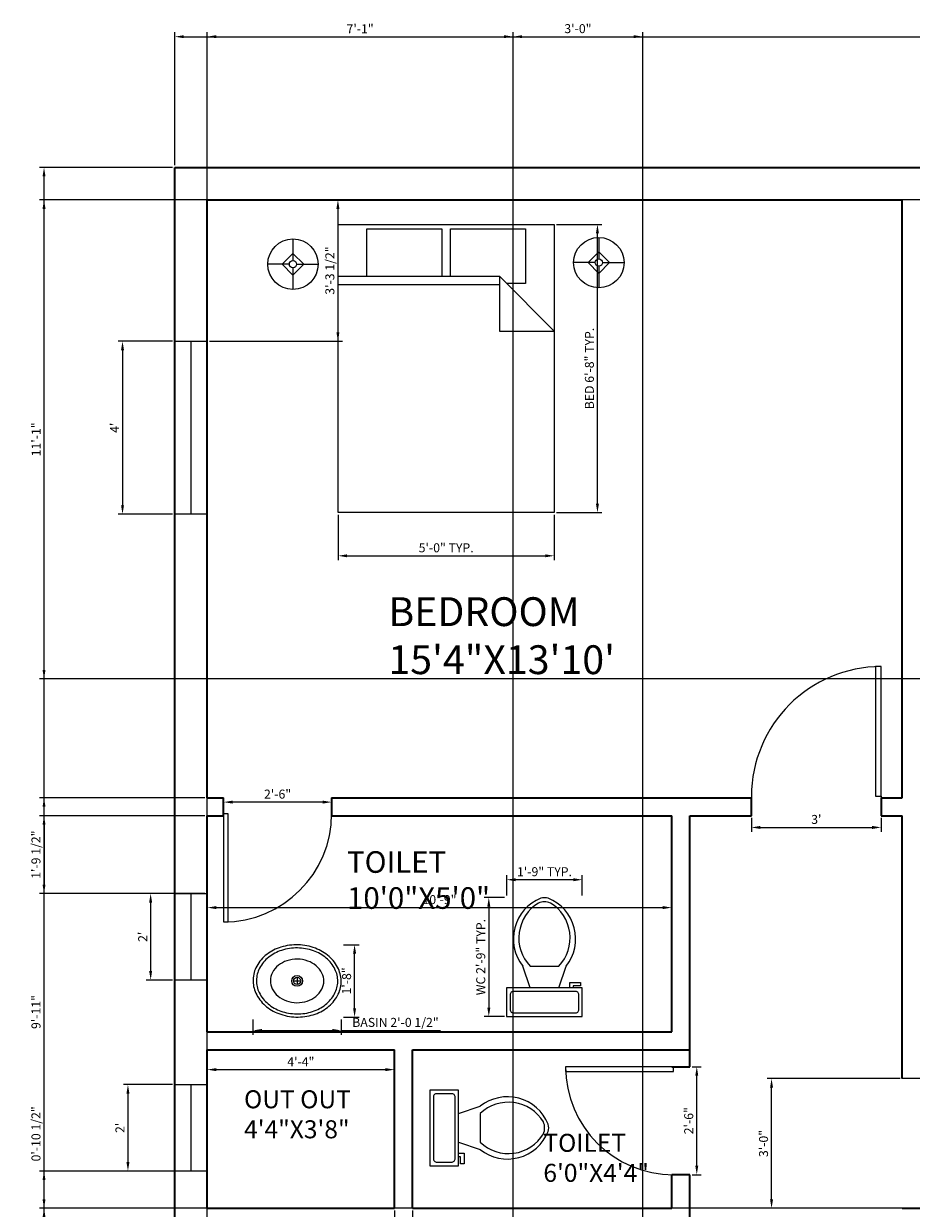
# Model space of a CAD drawing. Units: inches. Extents: x 3715 to 4224, y 2597 to 3354.
# Tile 4 of 5: x 3715 to 3961, y 3023 to 3352. Entities that reach past the tile are written whole.
import ezdxf

# ---------------------------------------------------------------- set-up
doc = ezdxf.new("R2010")
doc.units = ezdxf.units.IN
for name, color, linetype, lineweight in [('A-AREA-IDEN', 4, 'Continuous', 25), ('A-FLOR-FIXT', 9, 'Continuous', 18), ('A-WALL', 7, 'Continuous', 35), ('DIM', 1, 'Continuous', 18), ('DOOR', 3, 'Continuous', 25), ('FURNITURES', 30, 'Continuous', 18), ('WINDOW', 6, 'Continuous', 20)]:
    doc.layers.add(name, color=color, linetype=linetype, lineweight=lineweight)
doc.styles.get("Standard").update_dxf_attribs({"font": 'arial.ttf'})
doc.dimstyles.new('ISO-25', dxfattribs={"dimtxt": 2.5, "dimasz": 2.5, "dimexe": 1.25, "dimexo": 0.625, "dimtad": 1, "dimlunit": 3, "dimtxsty": 'Standard', "dimcen": 2.5, "dimadec": 0, "dimazin": 0, "dimtfac": 1, "dimtmove": 0, "dimatfit": 3, "dimfxl": 1, "dimarcsym": 0})

# ---------------------------------------------------------------- blocks, each defined once
blk = doc.blocks.new('*U4')
for p, q in [((0, 0), (0, -6)), ((-40, 0), (-40, -6))]:
    blk.add_line(p, q)
blk.add_lwpolyline([(0, 0), (0, 40), (-1.75, 40), (-1.75, 0)], close=True)
blk.add_arc((0, 0), 40, 90, 180)
blk = doc.blocks.new('*U5')
for p, q in [((0, 0), (0, 6)), ((40, 0), (40, 6))]:
    blk.add_line(p, q)
blk.add_lwpolyline([(0, 0), (0, -40), (1.75, -40), (1.75, 0)], close=True)
blk.add_arc((0, 0), 40, 270, 0)
blk = doc.blocks.new('Bed - Queen')
for p, q in [((0, -80.00003), (0, 0)), ((0, 0), (59.99999, 0)), ((59.99999, 0), (59.99999, -80.00003)), ((7.99999, -1.2), (28.79998, -1.2)), ((7.99999, -14.4), (7.99999, -1.2)), ((28.79998, -1.2), (28.79998, -14.4)), ((31.19999, -1.2), (51.99999, -1.2)), ((31.19999, -14.4), (31.19999, -1.2)), ((51.99999, -1.2), (51.99999, -16.4)), ((0, -14.4), (44.8, -14.4)), ((59.99999, -29.6), (44.8, -14.4)), ((44.8, -14.4), (44.8, -29.6)), ((51.99999, -16.4), (46.79936, -16.4)), ((44.8, -16.8), (0, -16.8)), ((44.8, -29.6), (59.99999, -29.6)), ((59.99999, -80.00003), (0, -80.00003))]:
    blk.add_line(p, q)
blk = doc.blocks.new('Lamp - Table')
for p, q in [((0, 7), (0, 1)), ((-1, 0), (-7, 0)), ((0, 3), (-3, 0)), ((-3, 0), (0, -3)), ((3, 0), (0, 3)), ((0, -3), (3, 0)), ((1, 0), (7, 0)), ((0, -1), (0, -7))]:
    blk.add_line(p, q)
for radius in [7, 1]:
    blk.add_circle((0, 0), radius)
blk = doc.blocks.new('Toilet - top')
for p, q in [((9.5, -6), (9.5, -2)), ((-10, -8.5), (-8, -8.5)), ((-10, -9.5), (-10, -8.5)), ((-7, -9.5), (-10, -9.5)), ((-8, -8.5), (-8, -8)), ((-7, -8), (-7, -9.5)), ((-4, -8), (-6, -14)), ((4, -8), (6, -14)), ((4, -14), (-4, -14))]:
    blk.add_line(p, q)
blk.add_lwpolyline([(10.5, -8), (10.5, 0), (-10.5, 0), (-10.5, -8)], close=True)
for points in [[(-9.5, -2), (-9.5, -6)], [(8.5, -1), (-8.5, -1)], [(-8.5, -7), (8.5, -7)]]:
    blk.add_lwpolyline(points)
for centre, radius, start, end in [((-8.62, -1.88), 0.884, 81.8699, 188.1301), ((8.62, -1.88), 0.884, 351.8699, 98.1301), ((-8.62, -6.12), 0.884, 171.8699, 278.1301), ((8.62, -6.12), 0.884, 261.8699, 8.1301), ((3.52, -21.58), 12.17, 141.4691, 247.9714), ((4.2, -21.82), 11.33, 136.3677, 238.9468), ((-3.52, -21.58), 12.17, 292.0284, 38.5307), ((-4.2, -21.82), 11.33, 301.053, 43.6321), ((0, -27.88), 4, 245.7318, 294.2682), ((0, -29), 4, 254.8605, 285.1395)]:
    blk.add_arc(centre, radius, start, end)
blk = doc.blocks.new('Sink - Oval top')
for p, q in [((-1, 0), (1, 0)), ((0, 1), (0, -1))]:
    blk.add_line(p, q)
for points in [[(-12.23, 0.39, 0.117634), (-11.46, -3.36, 0.104469), (-8.88, -6.8, 0.090016), (-5.08, -9.07, 0.08192), (-0.32, -10.02, 0.08192), (4.49, -9.38, 0.090016), (8.42, -7.36, 0.104469), (11.22, -4.09, 0.117634), (12.23, -0.39, 0.117634), (11.46, 3.36, 0.104469), (8.88, 6.8, 0.090016), (5.08, 9.07, 0.08192), (0.32, 10.02, 0.08192), (-4.49, 9.38, 0.090016), (-8.42, 7.36, 0.104469), (-11.22, 4.09, 0.117634)], [(-11.29, 0.16, 0.118622), (-10.52, -3.25, 0.104678), (-8.07, -6.36, 0.089562), (-4.54, -8.37, 0.081185), (-0.13, -9.15, 0.081185), (4.3, -8.49, 0.089562), (7.89, -6.58, 0.104678), (10.42, -3.55, 0.118622), (11.29, -0.16, 0.118622), (10.52, 3.25, 0.104678), (8.07, 6.36, 0.089562), (4.54, 8.37, 0.081185), (0.13, 9.15, 0.081185), (-4.3, 8.49, 0.089562), (-7.89, 6.58, 0.104678), (-10.42, 3.55, 0.118622)], [(-7.42, 0.08, 0.118283), (-6.91, -2.17, 0.104607), (-5.29, -4.21, 0.089718), (-2.97, -5.53, 0.081436), (-0.07, -6.04, 0.081436), (2.84, -5.59, 0.089718), (5.2, -4.33, 0.104607), (6.86, -2.32, 0.118283), (7.42, -0.08, 0.118283), (6.91, 2.17, 0.104607), (5.29, 4.21, 0.089718), (2.97, 5.53, 0.081436), (0.07, 6.04, 0.081436), (-2.84, 5.59, 0.089718), (-5.2, 4.33, 0.104607), (-6.86, 2.32, 0.118283)]]:
    blk.add_lwpolyline(points, format="xyb", close=True)
for radius in [1.5, 1]:
    blk.add_circle((0, 0), radius)
blk = doc.blocks.new('*D22')
at = {"layer": 'Defpoints', "color": 0, "transparency": 16777216}
for p in [(3756.48, 3263.65), (3741.97, 3215.65), (3756.48, 3215.65)]:
    blk.add_point(p, dxfattribs=at)
at = {"layer": 'DIM', "color": 0, "lineweight": -2, "transparency": 16777216}
for p, q in [((3755.85, 3263.65), (3740.72, 3263.65)), ((3741.97, 3261.15), (3741.97, 3218.15)), ((3755.85, 3215.65), (3740.72, 3215.65))]:
    blk.add_line(p, q, dxfattribs=at)
at = {"layer": 'DIM', "color": 0, "transparency": 16777216}
for points in [[(3741.55, 3261.15), (3742.39, 3261.15), (3741.97, 3263.65)], [(3741.55, 3218.15), (3742.39, 3218.15), (3741.97, 3215.65)]]:
    blk.add_solid(points, dxfattribs=at)
at = {"layer": 'DIM', "color": 0, "transparency": 16777216, "insert": (3740.1, 3239.65), "char_height": 2.5, "attachment_point": 5, "rotation": 90}
blk.add_mtext("4'", dxfattribs=at)
blk = doc.blocks.new('*D23')
at = {"layer": 'Defpoints', "color": 0, "transparency": 16777216}
for p in [(3756.48, 3110.32), (3749.78, 3086.32), (3756.48, 3086.32)]:
    blk.add_point(p, dxfattribs=at)
at = {"layer": 'DIM', "color": 0, "lineweight": -2, "transparency": 16777216}
for p, q in [((3755.85, 3110.32), (3748.53, 3110.32)), ((3749.78, 3107.82), (3749.78, 3088.82)), ((3755.85, 3086.32), (3748.53, 3086.32))]:
    blk.add_line(p, q, dxfattribs=at)
at = {"layer": 'DIM', "color": 0, "transparency": 16777216}
for points in [[(3749.36, 3107.82), (3750.19, 3107.82), (3749.78, 3110.32)], [(3749.36, 3088.82), (3750.19, 3088.82), (3749.78, 3086.32)]]:
    blk.add_solid(points, dxfattribs=at)
at = {"layer": 'DIM', "color": 0, "transparency": 16777216, "insert": (3747.9, 3098.32), "char_height": 2.5, "attachment_point": 5, "rotation": 90}
blk.add_mtext("2'", dxfattribs=at)
blk = doc.blocks.new('*D24')
at = {"layer": 'Defpoints', "color": 0, "transparency": 16777216}
for p in [(3756.48, 3057.27), (3743.47, 3033.27), (3756.48, 3033.27)]:
    blk.add_point(p, dxfattribs=at)
at = {"layer": 'DIM', "color": 0, "lineweight": -2, "transparency": 16777216}
for p, q in [((3755.85, 3057.27), (3742.22, 3057.27)), ((3743.47, 3054.77), (3743.47, 3035.77)), ((3755.85, 3033.27), (3742.22, 3033.27))]:
    blk.add_line(p, q, dxfattribs=at)
at = {"layer": 'DIM', "color": 0, "transparency": 16777216}
for points in [[(3743.06, 3054.77), (3743.89, 3054.77), (3743.47, 3057.27)], [(3743.06, 3035.77), (3743.89, 3035.77), (3743.47, 3033.27)]]:
    blk.add_solid(points, dxfattribs=at)
at = {"layer": 'DIM', "color": 0, "transparency": 16777216, "insert": (3741.59, 3045.27), "char_height": 2.5, "attachment_point": 5, "rotation": 90}
blk.add_mtext("2'", dxfattribs=at)
blk = doc.blocks.new('*D29')
at = {"layer": 'Defpoints', "color": 0, "transparency": 16777216}
for p in [(3765.48, 3066.93), (3817.48, 3064.87), (3817.48, 3061.44)]:
    blk.add_point(p, dxfattribs=at)
at = {"layer": 'DIM', "color": 0, "lineweight": -2, "transparency": 16777216}
for p, q in [((3765.48, 3066.31), (3765.48, 3060.19)), ((3817.48, 3064.25), (3817.48, 3060.19)), ((3767.98, 3061.44), (3814.98, 3061.44))]:
    blk.add_line(p, q, dxfattribs=at)
at = {"layer": 'DIM', "color": 0, "transparency": 16777216}
for points in [[(3767.98, 3061.86), (3767.98, 3061.02), (3765.48, 3061.44)], [(3814.98, 3061.86), (3814.98, 3061.02), (3817.48, 3061.44)]]:
    blk.add_solid(points, dxfattribs=at)
at = {"layer": 'DIM', "color": 0, "transparency": 16777216, "insert": (3791.48, 3063.31), "char_height": 2.5, "attachment_point": 5}
blk.add_mtext('4\'-4"', dxfattribs=at)
blk = doc.blocks.new('*D30')
at = {"layer": 'Defpoints', "color": 0, "transparency": 16777216}
for p in [(3894.48, 3106.42), (3765.48, 3071.93), (3894.48, 3071.93)]:
    blk.add_point(p, dxfattribs=at)
at = {"layer": 'DIM', "color": 0, "lineweight": -2, "transparency": 16777216}
for p, q in [((3765.48, 3072.56), (3765.48, 3107.67)), ((3767.98, 3106.42), (3891.98, 3106.42)), ((3894.48, 3072.56), (3894.48, 3107.67))]:
    blk.add_line(p, q, dxfattribs=at)
at = {"layer": 'DIM', "color": 0, "transparency": 16777216}
for points in [[(3767.98, 3106.84), (3767.98, 3106.01), (3765.48, 3106.42)], [(3891.98, 3106.84), (3891.98, 3106.01), (3894.48, 3106.42)]]:
    blk.add_solid(points, dxfattribs=at)
at = {"layer": 'DIM', "color": 0, "transparency": 16777216, "insert": (3829.98, 3108.32), "char_height": 2.5, "attachment_point": 5}
blk.add_mtext('10\'-9"', dxfattribs=at)
blk = doc.blocks.new('*D31')
at = {"layer": 'Defpoints', "color": 0, "transparency": 16777216}
for p in [(3916.6, 3131.93), (3952.6, 3131.93), (3952.6, 3128.68)]:
    blk.add_point(p, dxfattribs=at)
at = {"layer": 'DIM', "color": 0, "lineweight": -2, "transparency": 16777216}
for p, q in [((3916.6, 3131.31), (3916.6, 3127.43)), ((3952.6, 3131.31), (3952.6, 3127.43)), ((3919.1, 3128.68), (3950.1, 3128.68))]:
    blk.add_line(p, q, dxfattribs=at)
at = {"layer": 'DIM', "color": 0, "transparency": 16777216}
for points in [[(3919.1, 3129.1), (3919.1, 3128.26), (3916.6, 3128.68)], [(3950.1, 3129.1), (3950.1, 3128.26), (3952.6, 3128.68)]]:
    blk.add_solid(points, dxfattribs=at)
at = {"layer": 'DIM', "color": 0, "transparency": 16777216, "insert": (3934.6, 3130.58), "char_height": 2.5, "attachment_point": 5}
blk.add_mtext("3'", dxfattribs=at)
blk = doc.blocks.new('*D38')
at = {"layer": 'Defpoints', "color": 0, "transparency": 16777216}
for p in [(3899.48, 3062.26), (3901.41, 3062.26), (3899.48, 3032.26)]:
    blk.add_point(p, dxfattribs=at)
at = {"layer": 'DIM', "color": 0, "lineweight": -2, "transparency": 16777216}
for p, q in [((3900.1, 3062.26), (3902.66, 3062.26)), ((3901.41, 3034.76), (3901.41, 3059.76)), ((3900.1, 3032.26), (3902.66, 3032.26))]:
    blk.add_line(p, q, dxfattribs=at)
at = {"layer": 'DIM', "color": 0, "transparency": 16777216}
for points in [[(3900.99, 3059.76), (3901.82, 3059.76), (3901.41, 3062.26)], [(3900.99, 3034.76), (3901.82, 3034.76), (3901.41, 3032.26)]]:
    blk.add_solid(points, dxfattribs=at)
at = {"layer": 'DIM', "color": 0, "transparency": 16777216, "insert": (3899.5, 3047.26), "char_height": 2.5, "attachment_point": 5, "rotation": 90}
blk.add_mtext('2\'-6"', dxfattribs=at)
blk = doc.blocks.new('*D39')
at = {"layer": 'Defpoints', "color": 0, "transparency": 16777216}
for p in [(3770.02, 3136.93), (3770.02, 3135.71), (3800.02, 3136.93)]:
    blk.add_point(p, dxfattribs=at)
at = {"layer": 'DIM', "color": 0, "lineweight": -2, "transparency": 16777216}
for p, q in [((3770.02, 3136.31), (3770.02, 3134.46)), ((3797.52, 3135.71), (3772.52, 3135.71)), ((3800.02, 3136.31), (3800.02, 3134.46))]:
    blk.add_line(p, q, dxfattribs=at)
at = {"layer": 'DIM', "color": 0, "transparency": 16777216}
for points in [[(3772.52, 3136.13), (3772.52, 3135.3), (3770.02, 3135.71)], [(3797.52, 3136.13), (3797.52, 3135.3), (3800.02, 3135.71)]]:
    blk.add_solid(points, dxfattribs=at)
at = {"layer": 'DIM', "color": 0, "transparency": 16777216, "insert": (3785.02, 3137.61), "char_height": 2.5, "attachment_point": 5}
blk.add_mtext('2\'-6"', dxfattribs=at)
blk = doc.blocks.new('WIN-48IN-9IN-WALL')
blk.add_line((4.5, 48), (4.5, 0))
blk.add_lwpolyline([(0, 48), (9, 48), (9, 0), (0, 0)], close=True)
blk = doc.blocks.new('WIN-24IN-9IN-WALL')
blk.add_line((0, 4.5), (24, 4.5))
blk.add_lwpolyline([(0, 0), (0, 9), (24, 9), (24, 0)], close=True)
blk = doc.blocks.new('*D51')
at = {"layer": 'Defpoints', "color": 0, "transparency": 16777216}
for p in [(3861.83, 3296.1), (3873.83, 3296.1), (3861.83, 3216.1)]:
    blk.add_point(p, dxfattribs=at)
at = {"layer": 'DIM', "color": 0, "lineweight": -2, "transparency": 16777216}
for p, q in [((3862.46, 3296.1), (3875.08, 3296.1)), ((3873.83, 3218.6), (3873.83, 3293.6)), ((3862.46, 3216.1), (3875.08, 3216.1))]:
    blk.add_line(p, q, dxfattribs=at)
at = {"layer": 'DIM', "color": 0, "transparency": 16777216}
for points in [[(3873.41, 3293.6), (3874.25, 3293.6), (3873.83, 3296.1)], [(3873.41, 3218.6), (3874.25, 3218.6), (3873.83, 3216.1)]]:
    blk.add_solid(points, dxfattribs=at)
at = {"layer": 'DIM', "color": 0, "transparency": 16777216, "insert": (3871.93, 3256.1), "char_height": 2.5, "attachment_point": 5, "rotation": 90}
blk.add_mtext('BED 6\'-8" TYP.', dxfattribs=at)
blk = doc.blocks.new('*D52')
at = {"layer": 'Defpoints', "color": 0, "transparency": 16777216}
for p in [(3801.83, 3216.1), (3861.83, 3216.1), (3861.83, 3204.1)]:
    blk.add_point(p, dxfattribs=at)
at = {"layer": 'DIM', "color": 0, "lineweight": -2, "transparency": 16777216}
for p, q in [((3801.83, 3215.47), (3801.83, 3202.85)), ((3861.83, 3215.47), (3861.83, 3202.85)), ((3804.33, 3204.1), (3859.33, 3204.1))]:
    blk.add_line(p, q, dxfattribs=at)
at = {"layer": 'DIM', "color": 0, "transparency": 16777216}
for points in [[(3804.33, 3204.51), (3804.33, 3203.68), (3801.83, 3204.1)], [(3859.33, 3204.51), (3859.33, 3203.68), (3861.83, 3204.1)]]:
    blk.add_solid(points, dxfattribs=at)
at = {"layer": 'DIM', "color": 0, "transparency": 16777216, "insert": (3831.83, 3206), "char_height": 2.5, "attachment_point": 5}
blk.add_mtext('5\'-0" TYP.', dxfattribs=at)
blk = doc.blocks.new('*D55')
at = {"layer": 'Defpoints', "color": 0, "transparency": 16777216}
for p in [(3848.63, 3109.21), (3843.67, 3076.16), (3848.63, 3076.16)]:
    blk.add_point(p, dxfattribs=at)
at = {"layer": 'DIM', "color": 0, "lineweight": -2, "transparency": 16777216}
for p, q in [((3848, 3109.21), (3842.42, 3109.21)), ((3843.67, 3106.71), (3843.67, 3078.66)), ((3848, 3076.16), (3842.42, 3076.16))]:
    blk.add_line(p, q, dxfattribs=at)
at = {"layer": 'DIM', "color": 0, "transparency": 16777216}
for points in [[(3843.25, 3106.71), (3844.09, 3106.71), (3843.67, 3109.21)], [(3843.25, 3078.66), (3844.09, 3078.66), (3843.67, 3076.16)]]:
    blk.add_solid(points, dxfattribs=at)
at = {"layer": 'DIM', "color": 0, "transparency": 16777216, "insert": (3841.75, 3092.68), "char_height": 2.5, "attachment_point": 5, "rotation": 90}
blk.add_mtext('WC 2\'-9" TYP.', dxfattribs=at)
blk = doc.blocks.new('*D56')
at = {"layer": 'Defpoints', "color": 0, "transparency": 16777216}
for p in [(3848.63, 3114.16), (3848.63, 3109.21), (3869.63, 3109.21)]:
    blk.add_point(p, dxfattribs=at)
at = {"layer": 'DIM', "color": 0, "lineweight": -2, "transparency": 16777216}
for p, q in [((3848.63, 3109.83), (3848.63, 3115.41)), ((3869.63, 3109.83), (3869.63, 3115.41)), ((3867.13, 3114.16), (3851.13, 3114.16))]:
    blk.add_line(p, q, dxfattribs=at)
at = {"layer": 'DIM', "color": 0, "transparency": 16777216}
for points in [[(3851.13, 3114.58), (3851.13, 3113.75), (3848.63, 3114.16)], [(3867.13, 3114.58), (3867.13, 3113.75), (3869.63, 3114.16)]]:
    blk.add_solid(points, dxfattribs=at)
at = {"layer": 'DIM', "color": 0, "transparency": 16777216, "insert": (3859.13, 3116.07), "char_height": 2.5, "attachment_point": 5}
blk.add_mtext('1\'-9" TYP.', dxfattribs=at)
blk = doc.blocks.new('*D73')
at = {"layer": 'Defpoints', "color": 0, "transparency": 16777216}
for p in [(3778.17, 3076), (3802.72, 3076), (3802.72, 3072.31)]:
    blk.add_point(p, dxfattribs=at)
at = {"layer": 'DIM', "color": 0, "lineweight": -2, "transparency": 16777216}
for p, q in [((3778.17, 3075.37), (3778.17, 3071.06)), ((3802.72, 3075.37), (3802.72, 3071.06)), ((3780.67, 3072.31), (3800.22, 3072.31)), ((3802.72, 3072.31), (3830.28, 3072.31))]:
    blk.add_line(p, q, dxfattribs=at)
at = {"layer": 'DIM', "color": 0, "transparency": 16777216}
for points in [[(3780.67, 3072.73), (3780.67, 3071.9), (3778.17, 3072.31)], [(3800.22, 3072.73), (3800.22, 3071.9), (3802.72, 3072.31)]]:
    blk.add_solid(points, dxfattribs=at)
at = {"layer": 'DIM', "color": 0, "transparency": 16777216, "insert": (3817.75, 3074.23), "char_height": 2.5, "attachment_point": 5}
blk.add_mtext('BASIN 2\'-0 1/2"', dxfattribs=at)
blk = doc.blocks.new('*D74')
at = {"layer": 'Defpoints', "color": 0, "transparency": 16777216}
for p in [(3802.72, 3096.13), (3806.4, 3096.13), (3802.72, 3076)]:
    blk.add_point(p, dxfattribs=at)
at = {"layer": 'DIM', "color": 0, "lineweight": -2, "transparency": 16777216}
for p, q in [((3803.34, 3096.13), (3807.65, 3096.13)), ((3806.4, 3078.5), (3806.4, 3093.63)), ((3803.34, 3076), (3807.65, 3076))]:
    blk.add_line(p, q, dxfattribs=at)
at = {"layer": 'DIM', "color": 0, "transparency": 16777216}
for points in [[(3805.98, 3093.63), (3806.82, 3093.63), (3806.4, 3096.13)], [(3805.98, 3078.5), (3806.82, 3078.5), (3806.4, 3076)]]:
    blk.add_solid(points, dxfattribs=at)
at = {"layer": 'DIM', "color": 0, "transparency": 16777216, "insert": (3804.5, 3086.07), "char_height": 2.5, "attachment_point": 5, "rotation": 90}
blk.add_mtext('1\'-8"', dxfattribs=at)
blk = doc.blocks.new('*D75')
at = {"layer": 'Defpoints', "color": 0, "transparency": 16777216}
for p in [(4185.48, 3348.23), (3756.48, 3311.93), (4185.48, 3311.93)]:
    blk.add_point(p, dxfattribs=at)
at = {"layer": 'DIM', "color": 0, "lineweight": -2, "transparency": 16777216}
for p, q in [((3756.48, 3312.56), (3756.48, 3349.48)), ((4185.48, 3312.56), (4185.48, 3349.48)), ((3758.98, 3348.23), (4182.98, 3348.23))]:
    blk.add_line(p, q, dxfattribs=at)
at = {"layer": 'DIM', "color": 0, "transparency": 16777216}
for points in [[(3758.98, 3348.65), (3758.98, 3347.82), (3756.48, 3348.23)], [(4182.98, 3348.65), (4182.98, 3347.82), (4185.48, 3348.23)]]:
    blk.add_solid(points, dxfattribs=at)
at = {"layer": 'DIM', "color": 0, "transparency": 16777216, "insert": (3970.98, 3350.14), "char_height": 2.5, "attachment_point": 5}
blk.add_mtext('35\'-9"', dxfattribs=at)
blk = doc.blocks.new('*D76')
at = {"layer": 'Defpoints', "color": 0, "transparency": 16777216}
for p in [(3720.18, 3311.93), (3756.48, 3311.93), (3756.48, 2634.93)]:
    blk.add_point(p, dxfattribs=at)
at = {"layer": 'DIM', "color": 0, "lineweight": -2, "transparency": 16777216}
for p, q in [((3755.85, 3311.93), (3718.93, 3311.93)), ((3720.18, 2637.43), (3720.18, 3309.43)), ((3755.85, 2634.93), (3718.93, 2634.93))]:
    blk.add_line(p, q, dxfattribs=at)
at = {"layer": 'DIM', "color": 0, "transparency": 16777216}
for points in [[(3719.76, 3309.43), (3720.59, 3309.43), (3720.18, 3311.93)], [(3719.76, 2637.43), (3720.59, 2637.43), (3720.18, 2634.93)]]:
    blk.add_solid(points, dxfattribs=at)
at = {"layer": 'DIM', "color": 0, "transparency": 16777216, "insert": (3718.27, 2973.43), "char_height": 2.5, "attachment_point": 5, "rotation": 90}
blk.add_mtext('56\'-5"', dxfattribs=at)
blk = doc.blocks.new('*D77')
at = {"layer": 'Defpoints', "color": 0, "transparency": 16777216}
for p in [(3720.18, 3302.93), (4118.48, 3302.93), (4118.48, 3169.93)]:
    blk.add_point(p, dxfattribs=at)
at = {"layer": 'DIM', "color": 0, "lineweight": -2, "transparency": 16777216}
for p, q in [((4117.85, 3302.93), (3718.93, 3302.93)), ((3720.18, 3172.43), (3720.18, 3300.43)), ((4117.85, 3169.93), (3718.93, 3169.93))]:
    blk.add_line(p, q, dxfattribs=at)
at = {"layer": 'DIM', "color": 0, "transparency": 16777216}
for points in [[(3719.76, 3300.43), (3720.59, 3300.43), (3720.18, 3302.93)], [(3719.76, 3172.43), (3720.59, 3172.43), (3720.18, 3169.93)]]:
    blk.add_solid(points, dxfattribs=at)
at = {"layer": 'DIM', "color": 0, "transparency": 16777216, "insert": (3718.3, 3236.43), "char_height": 2.5, "attachment_point": 5, "rotation": 90}
blk.add_mtext('11\'-1"', dxfattribs=at)
blk = doc.blocks.new('*D79')
at = {"layer": 'Defpoints', "color": 0, "transparency": 16777216}
for p in [(3720.18, 3136.93), (3765.48, 3136.93), (3765.48, 3017.93)]:
    blk.add_point(p, dxfattribs=at)
at = {"layer": 'DIM', "color": 0, "lineweight": -2, "transparency": 16777216}
for p, q in [((3764.85, 3136.93), (3718.93, 3136.93)), ((3720.18, 3020.43), (3720.18, 3134.43)), ((3764.85, 3017.93), (3718.93, 3017.93))]:
    blk.add_line(p, q, dxfattribs=at)
at = {"layer": 'DIM', "color": 0, "transparency": 16777216}
for points in [[(3719.76, 3134.43), (3720.59, 3134.43), (3720.18, 3136.93)], [(3719.76, 3020.43), (3720.59, 3020.43), (3720.18, 3017.93)]]:
    blk.add_solid(points, dxfattribs=at)
at = {"layer": 'DIM', "color": 0, "transparency": 16777216, "insert": (3718.27, 3077.43), "char_height": 2.5, "attachment_point": 5, "rotation": 90}
blk.add_mtext('9\'-11"', dxfattribs=at)
blk = doc.blocks.new('*D83')
at = {"layer": 'Defpoints', "color": 0, "transparency": 16777216}
for p in [(3850.41, 3348.23), (3765.48, 2833.93), (3850.41, 2833.93)]:
    blk.add_point(p, dxfattribs=at)
at = {"layer": 'DIM', "color": 0, "lineweight": -2, "transparency": 16777216}
for p, q in [((3765.48, 2834.56), (3765.48, 3349.48)), ((3850.41, 2834.56), (3850.41, 3349.48)), ((3767.98, 3348.23), (3847.91, 3348.23))]:
    blk.add_line(p, q, dxfattribs=at)
at = {"layer": 'DIM', "color": 0, "transparency": 16777216}
for points in [[(3767.98, 3348.65), (3767.98, 3347.82), (3765.48, 3348.23)], [(3847.91, 3348.65), (3847.91, 3347.82), (3850.41, 3348.23)]]:
    blk.add_solid(points, dxfattribs=at)
at = {"layer": 'DIM', "color": 0, "transparency": 16777216, "insert": (3807.94, 3350.11), "char_height": 2.5, "attachment_point": 5}
blk.add_mtext('7\'-1"', dxfattribs=at)
blk = doc.blocks.new('*D84')
at = {"layer": 'Defpoints', "color": 0, "transparency": 16777216}
for p in [(3886.41, 3348.23), (3850.41, 2833.93), (3886.41, 2833.93)]:
    blk.add_point(p, dxfattribs=at)
at = {"layer": 'DIM', "color": 0, "lineweight": -2, "transparency": 16777216}
for p, q in [((3850.41, 2834.56), (3850.41, 3349.48)), ((3886.41, 2834.56), (3886.41, 3349.48)), ((3852.91, 3348.23), (3883.91, 3348.23))]:
    blk.add_line(p, q, dxfattribs=at)
at = {"layer": 'DIM', "color": 0, "transparency": 16777216}
for points in [[(3852.91, 3348.65), (3852.91, 3347.82), (3850.41, 3348.23)], [(3883.91, 3348.65), (3883.91, 3347.82), (3886.41, 3348.23)]]:
    blk.add_solid(points, dxfattribs=at)
at = {"layer": 'DIM', "color": 0, "transparency": 16777216, "insert": (3868.41, 3350.14), "char_height": 2.5, "attachment_point": 5}
blk.add_mtext('3\'-0"', dxfattribs=at)
blk = doc.blocks.new('*D85')
at = {"layer": 'Defpoints', "color": 0, "transparency": 16777216}
for p in [(3817.48, 3022.93), (3822.48, 3022.93), (3822.48, 2598.63)]:
    blk.add_point(p, dxfattribs=at)
at = {"layer": 'DIM', "color": 0, "lineweight": -2, "transparency": 16777216}
for p, q in [((3817.48, 3022.31), (3817.48, 2597.38)), ((3822.48, 3022.31), (3822.48, 2597.38)), ((3814.98, 2598.63), (3812.48, 2598.63)), ((3817.48, 2598.63), (3822.48, 2598.63)), ((3824.98, 2598.63), (3835.37, 2598.63))]:
    blk.add_line(p, q, dxfattribs=at)
at = {"layer": 'DIM', "color": 0, "transparency": 16777216}
for points in [[(3814.98, 2599.05), (3814.98, 2598.22), (3817.48, 2598.63)], [(3824.98, 2599.05), (3824.98, 2598.22), (3822.48, 2598.63)]]:
    blk.add_solid(points, dxfattribs=at)
at = {"layer": 'DIM', "color": 0, "transparency": 16777216, "insert": (3831.42, 2600.54), "char_height": 2.5, "attachment_point": 5}
blk.add_mtext('0\'-5"', dxfattribs=at)
blk = doc.blocks.new('*D90')
at = {"layer": 'Defpoints', "color": 0, "transparency": 16777216}
for p in [(3720.18, 3022.93), (3963.48, 3022.93), (3963.48, 3001.93)]:
    blk.add_point(p, dxfattribs=at)
at = {"layer": 'DIM', "color": 0, "lineweight": -2, "transparency": 16777216}
for p, q in [((3962.85, 3022.93), (3718.93, 3022.93)), ((3720.18, 3004.43), (3720.18, 3020.43)), ((3962.85, 3001.93), (3718.93, 3001.93))]:
    blk.add_line(p, q, dxfattribs=at)
at = {"layer": 'DIM', "color": 0, "transparency": 16777216}
for points in [[(3719.76, 3020.43), (3720.59, 3020.43), (3720.18, 3022.93)], [(3719.76, 3004.43), (3720.59, 3004.43), (3720.18, 3001.93)]]:
    blk.add_solid(points, dxfattribs=at)
at = {"layer": 'DIM', "color": 0, "transparency": 16777216, "insert": (3718.27, 3012.43), "char_height": 2.5, "attachment_point": 5, "rotation": 90}
blk.add_mtext('1\'-9"', dxfattribs=at)
blk = doc.blocks.new('*D91')
at = {"layer": 'Defpoints', "color": 0, "transparency": 16777216}
for p in [(3922.18, 3058.93), (3958.48, 3058.93), (3958.48, 3022.93)]:
    blk.add_point(p, dxfattribs=at)
at = {"layer": 'DIM', "color": 0, "lineweight": -2, "transparency": 16777216}
for p, q in [((3957.85, 3058.93), (3920.93, 3058.93)), ((3922.18, 3025.43), (3922.18, 3056.43)), ((3957.85, 3022.93), (3920.93, 3022.93))]:
    blk.add_line(p, q, dxfattribs=at)
at = {"layer": 'DIM', "color": 0, "transparency": 16777216}
for points in [[(3921.76, 3056.43), (3922.59, 3056.43), (3922.18, 3058.93)], [(3921.76, 3025.43), (3922.59, 3025.43), (3922.18, 3022.93)]]:
    blk.add_solid(points, dxfattribs=at)
at = {"layer": 'DIM', "color": 0, "transparency": 16777216, "insert": (3920.27, 3040.93), "char_height": 2.5, "attachment_point": 5, "rotation": 90}
blk.add_mtext('3\'-0"', dxfattribs=at)
blk = doc.blocks.new('*D97')
at = {"layer": 'Defpoints', "color": 0, "transparency": 16777216}
for p in [(3765.48, 3131.93), (3720.18, 3110.32), (3765.48, 3110.32)]:
    blk.add_point(p, dxfattribs=at)
at = {"layer": 'DIM', "color": 0, "lineweight": -2, "transparency": 16777216}
for p, q in [((3764.85, 3131.93), (3718.93, 3131.93)), ((3720.18, 3129.43), (3720.18, 3112.82)), ((3764.85, 3110.32), (3718.93, 3110.32))]:
    blk.add_line(p, q, dxfattribs=at)
at = {"layer": 'DIM', "color": 0, "transparency": 16777216}
for points in [[(3719.76, 3129.43), (3720.59, 3129.43), (3720.18, 3131.93)], [(3719.76, 3112.82), (3720.59, 3112.82), (3720.18, 3110.32)]]:
    blk.add_solid(points, dxfattribs=at)
at = {"layer": 'DIM', "color": 0, "transparency": 16777216, "insert": (3718.26, 3121.12), "char_height": 2.5, "attachment_point": 5, "rotation": 90}
blk.add_mtext('1\'-9 1/2"', dxfattribs=at)
blk = doc.blocks.new('*D98')
at = {"layer": 'Defpoints', "color": 0, "transparency": 16777216}
for p in [(3720.18, 3033.27), (3765.48, 3033.27), (3765.48, 3022.93)]:
    blk.add_point(p, dxfattribs=at)
at = {"layer": 'DIM', "color": 0, "lineweight": -2, "transparency": 16777216}
for p, q in [((3720.18, 3033.27), (3720.18, 3051.43)), ((3764.85, 3033.27), (3718.93, 3033.27)), ((3720.18, 3025.43), (3720.18, 3030.77)), ((3764.85, 3022.93), (3718.93, 3022.93))]:
    blk.add_line(p, q, dxfattribs=at)
at = {"layer": 'DIM', "color": 0, "transparency": 16777216}
for points in [[(3719.76, 3030.77), (3720.59, 3030.77), (3720.18, 3033.27)], [(3719.76, 3025.43), (3720.59, 3025.43), (3720.18, 3022.93)]]:
    blk.add_solid(points, dxfattribs=at)
at = {"layer": 'DIM', "color": 0, "transparency": 16777216, "insert": (3718.26, 3043.6), "char_height": 2.5, "attachment_point": 5, "rotation": 90}
blk.add_mtext('0\'-10 1/2"', dxfattribs=at)
blk = doc.blocks.new('*D100')
at = {"layer": 'Defpoints', "color": 0, "transparency": 16777216}
for p in [(3765.48, 3302.93), (3765.48, 3263.65), (3801.78, 3263.65)]:
    blk.add_point(p, dxfattribs=at)
at = {"layer": 'DIM', "color": 0, "lineweight": -2, "transparency": 16777216}
for p, q in [((3766.1, 3302.93), (3803.03, 3302.93)), ((3801.78, 3300.43), (3801.78, 3266.15)), ((3766.1, 3263.65), (3803.03, 3263.65))]:
    blk.add_line(p, q, dxfattribs=at)
at = {"layer": 'DIM', "color": 0, "transparency": 16777216}
for points in [[(3801.36, 3300.43), (3802.19, 3300.43), (3801.78, 3302.93)], [(3801.36, 3266.15), (3802.19, 3266.15), (3801.78, 3263.65)]]:
    blk.add_solid(points, dxfattribs=at)
at = {"layer": 'DIM', "color": 0, "transparency": 16777216, "insert": (3799.86, 3283.29), "char_height": 2.5, "attachment_point": 5, "rotation": 90}
blk.add_mtext('3\'-3 1/2"', dxfattribs=at)

msp = doc.modelspace()

# ---------------------------------------------------------------- linework, layer by layer
at = {"layer": 'A-WALL'}
for p, q in [((3756.476, 2634.934), (3756.476, 3311.934)), ((3756.476, 3311.934), (4185.476, 3311.934)), ((3765.476, 3302.934), (3958.476, 3302.934)), ((3765.476, 3136.934), (3765.476, 3302.934)), ((3958.476, 3136.934), (3958.476, 3302.934)), ((3765.476, 3136.934), (3770.02, 3136.934)), ((3800.02, 3136.934), (3916.604, 3136.934)), ((3952.604, 3136.934), (3958.476, 3136.934)), ((3765.476, 3131.934), (3770.02, 3131.934)), ((3765.476, 3071.934), (3765.476, 3131.934)), ((3800.02, 3131.934), (3894.476, 3131.934)), ((3894.476, 3071.934), (3894.476, 3131.934)), ((3899.476, 3062.26), (3899.476, 3131.934)), ((3899.476, 3131.934), (3916.604, 3131.934)), ((3952.604, 3131.934), (3958.476, 3131.934)), ((3958.476, 3058.934), (3958.476, 3131.934)), ((3765.476, 3071.934), (3894.476, 3071.934)), ((3765.476, 3066.934), (3817.476, 3066.934)), ((3765.476, 3022.934), (3765.476, 3066.934)), ((3817.476, 3022.934), (3817.476, 3066.934)), ((3822.476, 3022.934), (3822.476, 3066.934)), ((3822.476, 3066.934), (3899.476, 3066.934)), ((3894.476, 3022.934), (3894.476, 3032.26)), ((3899.476, 3017.934), (3899.476, 3032.26)), ((3765.476, 3022.934), (3817.476, 3022.934)), ((3822.476, 3022.934), (3894.476, 3022.934)), ((3958.476, 3022.934), (3963.476, 3022.934))]:
    msp.add_line(p, q, dxfattribs=at)
for points in [[(3770.02, 3131.934), (3770.02, 3136.934)], [(3800.02, 3136.934), (3800.02, 3131.934)], [(3916.604, 3131.934), (3916.604, 3136.934)], [(3952.604, 3136.934), (3952.604, 3131.934)], [(3894.476, 3062.26), (3899.476, 3062.26)], [(3899.476, 3032.26), (3894.476, 3032.26)]]:
    msp.add_lwpolyline(points, dxfattribs=at)

# ---------------------------------------------------------------- block references
at = {"layer": 'A-FLOR-FIXT'}
for p, rotation in [((3859.126, 3076.161), 180), ((3827.296, 3045.259), 89.99999999999999)]:
    msp.add_blockref('Toilet - top', p, dxfattribs=dict(at, rotation=rotation))
msp.add_blockref('Sink - Oval top', (3790.441, 3086.066), dxfattribs=at)
at = {"layer": 'DOOR'}
for name, p, xscale, yscale, zscale in [('*U4', (3952.604, 3137.334), 0.9, 0.9, 0.9), ('*U5', (3770.02, 3132.434), 0.75, 0.75, 0.75)]:
    msp.add_blockref(name, p, dxfattribs=dict(at, xscale=xscale, yscale=yscale, zscale=zscale))
for p, xscale, yscale, zscale, rotation in [((3894.976, 3062.26), 0.75, 0.75, 0.75, 90), ((3963.876, 3022.934), 0.9, 0.9, 0.9, 270)]:
    msp.add_blockref('*U4', p, dxfattribs=dict(at, xscale=xscale, yscale=yscale, zscale=zscale, rotation=rotation))
at = {"layer": 'FURNITURES'}
for name, p in [('Bed - Queen', (3801.832, 3296.096)), ('Lamp - Table', (3874.217, 3285.509)), ('Lamp - Table', (3789.286, 3285.062))]:
    msp.add_blockref(name, p, dxfattribs=at)
at = {"layer": 'WINDOW'}
msp.add_blockref('WIN-48IN-9IN-WALL', (3756.476, 3215.654), dxfattribs=at)
for p, rotation in [((3756.476, 3110.315), 269.999999999995), ((3756.476, 3057.27), 269.9999999999962)]:
    msp.add_blockref('WIN-24IN-9IN-WALL', p, dxfattribs=dict(at, rotation=rotation))

# ---------------------------------------------------------------- texts
at = {"layer": 'A-AREA-IDEN', "attachment_point": 1}
for s, insert, char_height in [('BEDROOM\\P15\'4"X13\'10\'', (3815.789, 3192.586), 8), ('TOILET\\P10\'0"X5\'0"', (3804.294, 3122.081), 6), ('OUT OUT\\P4\'4"X3\'8"', (3775.709, 3055.704), 5), ('TOILET\\P6\'0"X4\'4"', (3858.819, 3043.615), 5)]:
    msp.add_mtext_dynamic_manual_height_columns(s, width=94.29963, gutter_width=12.5, heights=[0], dxfattribs=dict(at, insert=insert, char_height=char_height))

# ---------------------------------------------------------------- dimensions: what is measured, and where the dimension line sits
at = {"layer": 'DIM'}
for base, p1, p2, override, picture, middle in [((4185.476, 3348.234), (3756.476, 3311.934), (4185.476, 3311.934), {"dimdec": 1, "dimlfac": 1, "dimrnd": 0, "dimzin": 1, "dimdsep": 46, "dimlunit": 4, "dimfrac": 2}, '*D75', (3970.976, 3350.136)), ((3850.407, 3348.234), (3765.476, 2833.934), (3850.407, 2833.934), {"dimdec": 1, "dimlfac": 1, "dimrnd": 0, "dimzin": 1, "dimdsep": 46, "dimlunit": 4, "dimfrac": 2}, '*D83', (3807.941, 3350.114)), ((3886.407, 3348.234), (3850.407, 2833.934), (3886.407, 2833.934), {"dimdec": 1, "dimlfac": 1, "dimrnd": 0, "dimzin": 1, "dimdsep": 46, "dimlunit": 4, "dimfrac": 2}, '*D84', (3868.407, 3350.136)), ((3770.02, 3135.713), (3800.02, 3136.934), (3770.02, 3136.934), {"dimclrd": 0, "dimclre": 0, "dimclrt": 0}, '*D39', (3785.02, 3137.614)), ((3952.604, 3128.68), (3916.604, 3131.934), (3952.604, 3131.934), {"dimclrd": 0, "dimclre": 0, "dimclrt": 0}, '*D31', (3934.604, 3130.582)), ((3894.476, 3106.422), (3765.476, 3071.934), (3894.476, 3071.934), {"dimclrd": 0, "dimclre": 0, "dimclrt": 0}, '*D30', (3829.976, 3108.324)), ((3817.476, 3061.439), (3765.476, 3066.934), (3817.476, 3064.87), {"dimclrd": 0, "dimclre": 0, "dimclrt": 0}, '*D29', (3791.476, 3063.314)), ((3822.476, 2598.634), (3817.476, 3022.934), (3822.476, 3022.934), {"dimdec": 1, "dimlfac": 1, "dimrnd": 0, "dimzin": 1, "dimdsep": 46, "dimlunit": 4, "dimfrac": 2}, '*D85', (3831.423, 2600.535))]:
    dim = msp.add_linear_dim(base=base, p1=p1, p2=p2, dimstyle='ISO-25', override=override, dxfattribs=at)
    dim.commit()
    dim.dimension.update_dxf_attribs({"geometry": picture, "text_midpoint": middle})
for base, p1, p2, angle, override, picture, middle in [((3720.176, 3311.934), (3756.476, 2634.934), (3756.476, 3311.934), 90, {"dimdec": 1, "dimlfac": 1, "dimrnd": 0, "dimzin": 1, "dimdsep": 46, "dimlunit": 4, "dimfrac": 2}, '*D76', (3718.274, 2973.434)), ((3720.176, 3302.934), (4118.476, 3169.934), (4118.476, 3302.934), 90, {"dimdec": 1, "dimlfac": 1, "dimrnd": 0, "dimzin": 1, "dimdsep": 46, "dimlunit": 4, "dimfrac": 2}, '*D77', (3718.295, 3236.434)), ((3801.776, 3263.654), (3765.476, 3302.934), (3765.476, 3263.654), 270, {"dimdec": 1, "dimlfac": 1, "dimrnd": 0, "dimzin": 1, "dimdsep": 46, "dimlunit": 4, "dimfrac": 2}, '*D100', (3799.857, 3283.294)), ((3741.971, 3215.654), (3756.476, 3263.654), (3756.476, 3215.654), 90, {"dimclrd": 0, "dimclre": 0, "dimclrt": 0}, '*D22', (3740.096, 3239.654)), ((3720.176, 3136.934), (3765.476, 3017.934), (3765.476, 3136.934), 90, {"dimdec": 1, "dimlfac": 1, "dimrnd": 0, "dimzin": 1, "dimdsep": 46, "dimlunit": 4, "dimfrac": 2}, '*D79', (3718.274, 3077.434)), ((3720.176, 3110.316), (3765.476, 3131.934), (3765.476, 3110.316), 90, {"dimdec": 1, "dimlfac": 1, "dimrnd": 0, "dimzin": 1, "dimdsep": 46, "dimlunit": 4, "dimfrac": 2}, '*D97', (3718.258, 3121.125)), ((3749.778, 3086.316), (3756.476, 3110.316), (3756.476, 3086.316), 90, {"dimclrd": 0, "dimclre": 0, "dimclrt": 0}, '*D23', (3747.898, 3098.316)), ((3806.399, 3096.134), (3802.716, 3075.997), (3802.716, 3096.134), 90, {"dimdec": 1, "dimlfac": 1, "dimrnd": 0, "dimzin": 1, "dimdsep": 46, "dimlunit": 4, "dimfrac": 2}, '*D74', (3804.497, 3086.066)), ((3901.406, 3062.26), (3899.476, 3032.26), (3899.476, 3062.26), 90, {"dimclrd": 0, "dimclre": 0, "dimclrt": 0}, '*D38', (3899.504, 3047.26)), ((3922.176, 3058.934), (3958.476, 3022.934), (3958.476, 3058.934), 90, {"dimdec": 1, "dimlfac": 1, "dimrnd": 0, "dimzin": 1, "dimdsep": 46, "dimlunit": 4, "dimfrac": 2}, '*D91', (3920.273, 3040.934)), ((3743.473, 3033.27), (3756.476, 3057.27), (3756.476, 3033.27), 90, {"dimclrd": 0, "dimclre": 0, "dimclrt": 0}, '*D24', (3741.593, 3045.27)), ((3720.176, 3033.27), (3765.476, 3022.934), (3765.476, 3033.27), 90, {"dimdec": 1, "dimlfac": 1, "dimrnd": 0, "dimzin": 1, "dimdsep": 46, "dimlunit": 4, "dimfrac": 2}, '*D98', (3718.258, 3043.602)), ((3720.176, 3022.934), (3963.476, 3001.934), (3963.476, 3022.934), 90, {"dimdec": 1, "dimlfac": 1, "dimrnd": 0, "dimzin": 1, "dimdsep": 46, "dimlunit": 4, "dimfrac": 2}, '*D90', (3718.274, 3012.434))]:
    dim = msp.add_linear_dim(base=base, p1=p1, p2=p2, angle=angle, dimstyle='ISO-25', override=override, dxfattribs=at)
    dim.commit()
    dim.dimension.update_dxf_attribs({"geometry": picture, "text_midpoint": middle})
for base, p1, p2, angle, text, picture, middle in [((3873.832, 3296.096), (3861.832, 3216.095), (3861.832, 3296.096), 90, 'BED <> TYP.', '*D51', (3871.93, 3256.095)), ((3848.626, 3114.164), (3869.626, 3109.207), (3848.626, 3109.207), 180, '<> TYP.', '*D56', (3859.126, 3116.065)), ((3843.669, 3076.161), (3848.626, 3109.207), (3848.626, 3076.161), 270, 'WC <> TYP.', '*D55', (3841.751, 3092.684))]:
    dim = msp.add_linear_dim(base=base, p1=p1, p2=p2, angle=angle, text=text, dimstyle='ISO-25', override={"dimdec": 1, "dimlfac": 1, "dimrnd": 0, "dimzin": 1, "dimdsep": 46, "dimlunit": 4, "dimfrac": 2}, dxfattribs=at)
    dim.commit()
    dim.dimension.update_dxf_attribs({"geometry": picture, "text_midpoint": middle})
for base, p1, p2, text, picture, middle in [((3861.832, 3204.095), (3801.832, 3216.095), (3861.832, 3216.095), '<> TYP.', '*D52', (3831.832, 3205.997)), ((3802.716, 3072.315), (3778.165, 3075.997), (3802.716, 3075.997), 'BASIN <>', '*D73', (3817.747, 3074.232))]:
    dim = msp.add_linear_dim(base=base, p1=p1, p2=p2, text=text, dimstyle='ISO-25', override={"dimdec": 1, "dimlfac": 1, "dimrnd": 0, "dimzin": 1, "dimdsep": 46, "dimlunit": 4, "dimfrac": 2}, dxfattribs=at)
    dim.commit()
    dim.dimension.update_dxf_attribs({"geometry": picture, "text_midpoint": middle})

doc.saveas('drawing.dxf')
